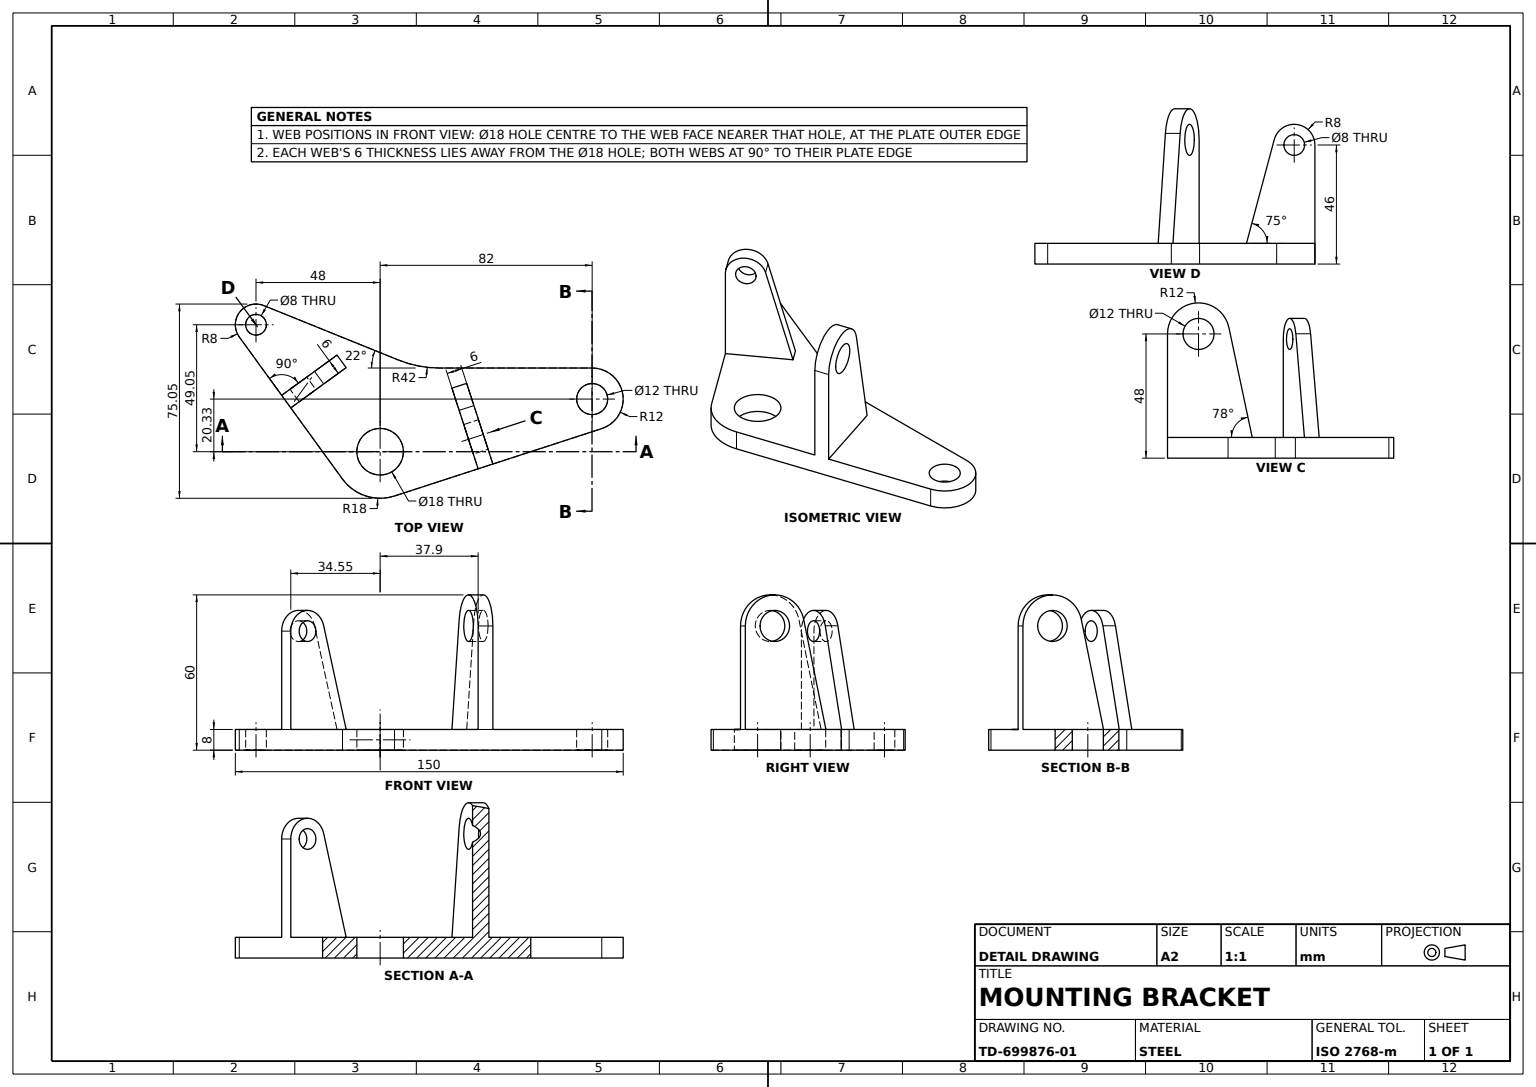
SolidWorks part; units mm, degrees
material "Plain Carbon Steel"
ref_plane "Front Plane" through (0, 0, 0) normal (0, 0, 1) x (1, 0, 0)
ref_plane "Top Plane" through (0, 0, 0) normal (0, 1, 0) x (1, 0, 0)
ref_plane "Right Plane" through (0, 0, 0) normal (1, 0, 0) x (0, 0, -1)
sketch "Base Plate Sketch" plane through (0, 0, 0) normal (0, 1, 0) x (1, 0, 0)
  line L0 (82, 32.3346) -> (22.8999, 32.3346)
  line L1 (85.7082, 8.922) -> (5.5623, -17.119)
  line L2 (-45.0031, 56.4708) -> (7.1664, 35.3929)
  line L3 (-54.4721, 44.351) -> (-14.5623, -10.5801)
  circle A0 centre (0, 0) radius 9
  arc A1 (-14.5623, -10.5801) -> (5.5623, -17.119) centre (0, 0) ccw
  arc A2 (85.7082, 8.922) -> (82, 32.3346) centre (82, 20.3346) ccw
  circle A3 centre (82, 20.3346) radius 6
  circle A4 centre (-48, 49.0533) radius 4
  arc A5 (-45.0031, 56.4708) -> (-54.4721, 44.351) centre (-48, 49.0533) ccw
  arc A6 (22.8999, 32.3346) -> (7.1664, 35.3929) centre (22.8999, 74.3346) cw
  dimension "D1" = 18
  dimension "D2" = 36
  dimension "D3" = 24
  dimension "D4" = 12
  dimension "D5" = 8
  dimension "D6" = 16
  dimension "D12" = 42
  dimension "D7" = 48
  dimension "D8" = 82
  dimension "D9" = 54
  dimension "D10" = 22
  dimension "D11" = 18
extrude "Base Plate" add sketch "Base Plate Sketch" along normal blind 8
sketch "Upright Web Sketch" plane through (0, 8, 0) normal (0, 1, 0) x (1, 0, 0)
  line L0 (-34.547, 16.9264) -> (-10.807, 34.1746)
  line L1 (-54.4721, 44.351) -> (-14.5623, -10.5801) construction
  line L2 (-10.807, 34.1746) -> (-14.3337, 39.0287)
  line L3 (-14.3337, 39.0287) -> (-38.0737, 21.7805)
  line L4 (-38.0737, 21.7805) -> (-34.547, 16.9264)
  line L5 (37.8982, -6.6124) -> (28.4561, 22.4474)
  line L6 (5.5623, -17.119) -> (85.7082, 8.922) construction
  line L7 (28.4561, 22.4474) -> (34.1624, 24.3015)
  line L8 (34.1624, 24.3015) -> (43.6046, -4.7583)
  line L9 (43.6046, -4.7583) -> (37.8982, -6.6124)
  line L10 (82, 32.3346) -> (22.8999, 32.3346) construction
  dimension "D1" = 90
  dimension "D2" = 6
  dimension "D3" = 34
  dimension "D4" = 6
  dimension "D5" = 34
  dimension "D6" = 40.1385
  dimension "D7" = 43.6652
  dimension "D8" = 82.9282
  dimension "D9" = 6.694
extrude "Upright Web" add sketch "Upright Web Sketch" along normal blind 98
sketch "Web Angled Trim Sketch" plane through (-23.5114, 0, -32.3607) normal (-0.5878, 0, -0.809) x (-0.809, 0, 0.5878)
  line L0 (-8.4643, 8) -> (2.2726, 48.0706)
  line L1 (-26.6012, 8) -> (3.2156, 8) construction
  line L2 (3.2156, 0) -> (18, 0) construction
  line L3 (18, 106) -> (18, 8) construction
  line L4 (-11.3443, 8) -> (18, 8) construction
  line L5 (-8.4643, 8) -> (-16.1387, 8)
  line L6 (-16.1387, 8) -> (-18.2797, 110.5495)
  line L7 (-18.2797, 110.5495) -> (48.4192, 110.5495)
  line L8 (48.4192, 110.5495) -> (24.0453, 43.3565)
  line L9 (24.0453, 43.3565) -> (18, 46)
  arc A0 (18, 46) -> (2.2726, 48.0706) centre (10, 46) ccw
  circle A1 centre (10, 46) radius 4
  dimension "D2" = 8
  dimension "D3" = 16
  dimension "D1" = 75
  dimension "D4" = 46
  dimension "D5" = 6.0453
  dimension "D6" = 30.4192
  dimension "D7" = 8
  dimension "D8" = 35.3565
  dimension "D9" = 102.5495
  dimension "D10" = 34.1387
  dimension "D11" = 36.2797
extrude "Web Angled Trim" cut sketch "Web Angled Trim Sketch" against normal blind 98
sketch "Pivot Lug Sketch" plane through (38.0423, 0, -12.3607) normal (0.9511, 0, -0.309) x (-0.309, 0, -0.9511)
  line L0 (14.7703, 8) -> (5.7378, 50.4949)
  line L1 (5.4127, 8) -> (23.6756, 8) construction
  line L2 (-18, 8) -> (-18, 48)
  line L4 (-18, 0) -> (5.4127, 0) construction
  line L5 (5.4127, 0) -> (23.6756, 0) construction
  line L6 (-18, 8) -> (14.7703, 8)
  arc A0 (5.7378, 50.4949) -> (-18, 48) centre (-6, 48) ccw
  circle A1 centre (-6, 48) radius 6
  dimension "D3" = 12
  dimension "D4" = 24
  dimension "D1" = 78
  dimension "D2" = 48
extrude "Pivot Lug" add sketch "Pivot Lug Sketch" against normal blind 6
sketch "Lug Cut Sketch" plane through (38.0423, 0, -12.3607) normal (0.9511, 0, -0.309) x (-0.309, 0, -0.9511)
  line L0 (-18, 106) -> (-18, 8) construction
  line L1 (-18, 8) -> (14.7703, 8) construction
  line L2 (12.5553, 18.4208) -> (5.7378, 50.4949)
  line L4 (-18, 0) -> (5.4127, 0) construction
  line L5 (-18, 48) -> (-46.798, 119.8219)
  line L6 (-46.798, 119.8219) -> (32.7221, 114.4556)
  line L7 (32.7221, 114.4556) -> (12.5553, 18.4208)
  arc A0 (5.7378, 50.4949) -> (-18, 48) centre (-6, 48) ccw
  circle A1 centre (-6, 48) radius 6
  dimension "D3" = 24
  dimension "D4" = 12
  dimension "D1" = 48
  dimension "D2" = 78
  dimension "D5" = 50.7221
  dimension "D6" = 28.798
  dimension "D7" = 106.4556
  dimension "D8" = 111.8219
extrude "Lug Cut" cut sketch "Lug Cut Sketch" against normal blind 16
